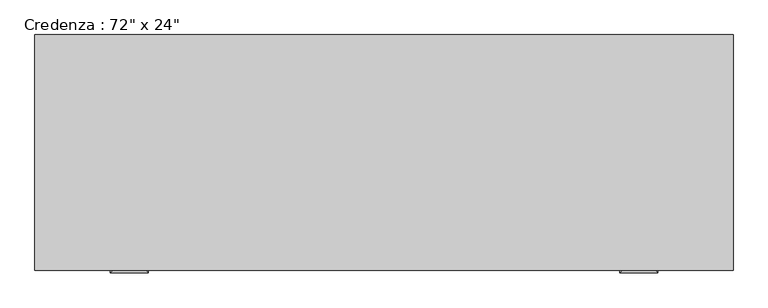
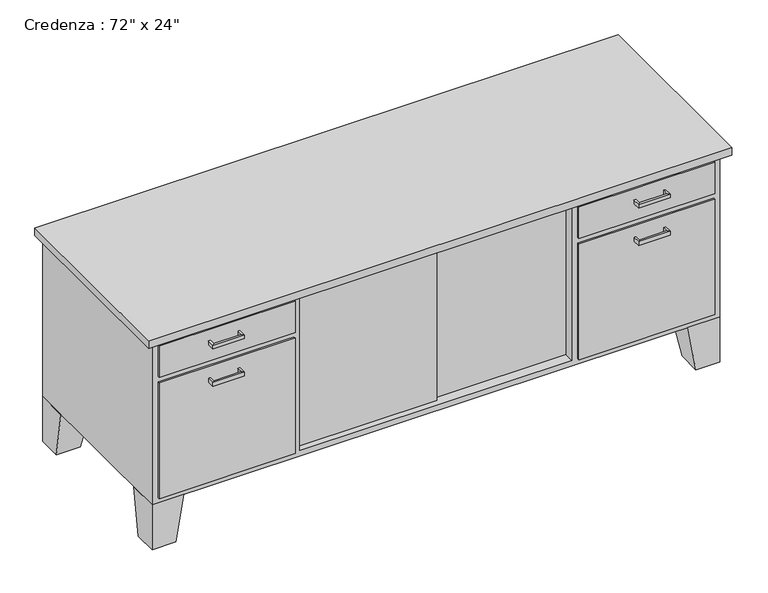
"""IFC4 building model written with IfcOpenShell, lengths in millimetres: furniture geometry."""

from ifc_helpers import new_model, si_unit, frame, origin, place, context, project, spatial, polyline, outline, extrude, faceted_brep, source, transform, mapped, element, save


def furniture_7b927048(model_context):
    return source(origin(), model_context, "Body", "SolidModel", [
        extrude(outline(polyline([(531.7023176, -267.2714583), (46.8442623, -267.2714583), (46.8442623, -254.5714583), (531.7023176, -254.5714583), (531.7023176, -267.2714583)])), frame((0.0, 0.0, 171.45), z_axis=(0.0, 0.0, 1.0), x_axis=(1.0, 0.0, 0.0)), (0.0, 0.0, 1.0), 520.7),
        extrude(outline(polyline([(73.6254475, -279.9714583), (-378.6057377, -279.9714583), (-378.6057377, -267.2714583), (73.6254475, -267.2714583), (73.6254475, -279.9714583)])), frame((0.0, 0.0, 171.45), z_axis=(0.0, 0.0, 1.0), x_axis=(1.0, 0.0, 0.0)), (0.0, 0.0, 1.0), 520.7),
        faceted_brep([(872.3442623, 309.3803279, 152.4), (872.3442623, 207.7803279, 152.4), (973.9442623, 207.7803279, 152.4), (973.9442623, 309.3803279, 152.4), (897.7442623, 309.3803279, 0.0), (973.9442623, 309.3803279, 0.0), (973.9442623, 233.1803279, 0.0), (897.7442623, 233.1803279, 0.0)], [[[0, 1, 2, 3]], [[4, 5, 6, 7]], [[4, 7, 1, 0]], [[7, 6, 2, 1]], [[6, 5, 3, 2]], [[5, 4, 0, 3]]]),
        extrude(outline(polyline([(954.8942623, -306.5696721), (516.7442623, -306.5696721), (516.7442623, -300.2196721), (954.8942623, -300.2196721), (954.8942623, -306.5696721)])), frame((0.0, 0.0, 584.2), z_axis=(0.0, 0.0, 1.0), x_axis=(1.0, 0.0, 0.0)), (0.0, 0.0, 1.0), 107.95),
        extrude(outline(polyline([(954.8942623, -306.5696721), (516.7442623, -306.5696721), (516.7442623, -300.2196721), (954.8942623, -300.2196721), (954.8942623, -306.5696721)])), frame((0.0, 0.0, 171.45), z_axis=(0.0, 0.0, 1.0), x_axis=(1.0, 0.0, 0.0)), (0.0, 0.0, 1.0), 393.7),
        extrude(outline(polyline([(-397.6557377, -306.5696721), (-835.8057377, -306.5696721), (-835.8057377, -300.2196721), (-397.6557377, -300.2196721), (-397.6557377, -306.5696721)])), frame((0.0, 0.0, 584.2), z_axis=(0.0, 0.0, 1.0), x_axis=(1.0, 0.0, 0.0)), (0.0, 0.0, 1.0), 107.95),
        extrude(outline(polyline([(-397.6557377, -306.5696721), (-835.8057377, -306.5696721), (-835.8057377, -300.2196721), (-397.6557377, -300.2196721), (-397.6557377, -306.5696721)])), frame((0.0, 0.0, 171.45), z_axis=(0.0, 0.0, 1.0), x_axis=(1.0, 0.0, 0.0)), (0.0, 0.0, 1.0), 393.7),
        faceted_brep([(-753.2557377, -300.2196721, 152.4), (-753.2557377, -198.6196721, 152.4), (-854.8557377, -198.6196721, 152.4), (-854.8557377, -300.2196721, 152.4), (-778.6557377, -300.2196721, 0.0), (-854.8557377, -300.2196721, 0.0), (-854.8557377, -224.0196721, 0.0), (-778.6557377, -224.0196721, 0.0)], [[[0, 1, 2, 3]], [[4, 5, 6, 7]], [[4, 7, 1, 0]], [[7, 6, 2, 1]], [[6, 5, 3, 2]], [[5, 4, 0, 3]]]),
        faceted_brep([(-753.2557377, 309.3803279, 152.4), (-854.8557377, 309.3803279, 152.4), (-854.8557377, 207.7803279, 152.4), (-753.2557377, 207.7803279, 152.4), (-778.6557377, 309.3803279, 0.0), (-778.6557377, 233.1803279, 0.0), (-854.8557377, 233.1803279, 0.0), (-854.8557377, 309.3803279, 0.0)], [[[0, 1, 2, 3]], [[4, 5, 6, 7]], [[4, 7, 1, 0]], [[7, 6, 2, 1]], [[6, 5, 3, 2]], [[5, 4, 0, 3]]]),
        faceted_brep([(872.3442623, -300.2196721, 152.4), (973.9442623, -300.2196721, 152.4), (973.9442623, -198.6196721, 152.4), (872.3442623, -198.6196721, 152.4), (897.7442623, -300.2196721, 0.0), (897.7442623, -224.0196721, 0.0), (973.9442623, -224.0196721, 0.0), (973.9442623, -300.2196721, 0.0)], [[[0, 1, 2, 3]], [[4, 5, 6, 7]], [[4, 7, 1, 0]], [[7, 6, 2, 1]], [[6, 5, 3, 2]], [[5, 4, 0, 3]]]),
        faceted_brep([(973.9442623, 309.3803279, 711.2), (-854.8557377, 309.3803279, 711.2), (-854.8557377, -300.2196721, 711.2), (973.9442623, -300.2196721, 711.2), (973.9442623, 309.3803279, 152.4), (973.9442623, -300.2196721, 152.4), (-854.8557377, -300.2196721, 152.4), (-854.8557377, 309.3803279, 152.4), (-378.6057377, -300.2196721, 692.15), (497.6942623, -300.2196721, 692.15), (497.6942623, -300.2196721, 171.45), (-378.6057377, -300.2196721, 171.45), (497.6942623, 290.3303279, 692.15), (-378.6057377, 290.3303279, 692.15), (-378.6057377, 290.3303279, 171.45), (497.6942623, 290.3303279, 171.45)], [[[0, 1, 2, 3]], [[4, 5, 6, 7]], [[1, 0, 4, 7]], [[2, 1, 7, 6]], [[3, 2, 6, 5], [8, 9, 10, 11]], [[0, 3, 5, 4]], [[12, 13, 14, 15]], [[13, 12, 9, 8]], [[14, 13, 8, 11]], [[15, 14, 11, 10]], [[12, 15, 10, 9]]]),
        extrude(outline(polyline([(999.3442623, 309.3803279), (999.3442623, -325.6196721), (-880.2557377, -325.6196721), (-880.2557377, 309.3803279), (999.3442623, 309.3803279)])), frame((0.0, 0.0, 711.2), z_axis=(0.0, 0.0, 1.0), x_axis=(1.0, 0.0, 0.0)), (0.0, 0.0, 1.0), 25.4),
        faceted_brep([(-670.7057377, -306.5696721, 527.05), (-670.7057377, -306.5696721, 514.35), (-677.0557377, -306.5696721, 514.35), (-677.0557377, -306.5696721, 527.05), (-670.7057377, -325.6196721, 527.05), (-670.7057377, -325.6196721, 514.35), (-677.0557377, -331.9696721, 514.35), (-677.0557377, -331.9696721, 527.05), (-581.8057377, -325.6196721, 527.05), (-581.8057377, -325.6196721, 514.35), (-575.4557377, -331.9696721, 514.35), (-575.4557377, -331.9696721, 527.05), (-581.8057377, -306.5696721, 527.05), (-575.4557377, -306.5696721, 527.05), (-575.4557377, -306.5696721, 514.35), (-581.8057377, -306.5696721, 514.35)], [[[0, 1, 2, 3]], [[1, 0, 4, 5]], [[2, 1, 5, 6]], [[3, 2, 6, 7]], [[0, 3, 7, 4]], [[5, 4, 8, 9]], [[6, 5, 9, 10]], [[7, 6, 10, 11]], [[4, 7, 11, 8]], [[12, 13, 14, 15]], [[9, 8, 12, 15]], [[10, 9, 15, 14]], [[11, 10, 14, 13]], [[8, 11, 13, 12]]]),
        faceted_brep([(-670.7057377, -306.5696721, 654.05), (-670.7057377, -306.5696721, 641.35), (-677.0557377, -306.5696721, 641.35), (-677.0557377, -306.5696721, 654.05), (-670.7057377, -325.6196721, 654.05), (-670.7057377, -325.6196721, 641.35), (-677.0557377, -331.9696721, 641.35), (-677.0557377, -331.9696721, 654.05), (-581.8057377, -325.6196721, 654.05), (-581.8057377, -325.6196721, 641.35), (-575.4557377, -331.9696721, 641.35), (-575.4557377, -331.9696721, 654.05), (-581.8057377, -306.5696721, 654.05), (-575.4557377, -306.5696721, 654.05), (-575.4557377, -306.5696721, 641.35), (-581.8057377, -306.5696721, 641.35)], [[[0, 1, 2, 3]], [[1, 0, 4, 5]], [[2, 1, 5, 6]], [[3, 2, 6, 7]], [[0, 3, 7, 4]], [[5, 4, 8, 9]], [[6, 5, 9, 10]], [[7, 6, 10, 11]], [[4, 7, 11, 8]], [[12, 13, 14, 15]], [[9, 8, 12, 15]], [[10, 9, 15, 14]], [[11, 10, 14, 13]], [[8, 11, 13, 12]]]),
        faceted_brep([(700.8942623, -306.5696721, 654.1373112), (700.8942623, -306.5696721, 641.4373112), (694.5442623, -306.5696721, 641.4373112), (694.5442623, -306.5696721, 654.1373112), (700.8942623, -325.6196721, 654.1373112), (700.8942623, -325.6196721, 641.4373112), (694.5442623, -331.9696721, 641.4373112), (694.5442623, -331.9696721, 654.1373112), (789.7942623, -325.6196721, 654.1373112), (789.7942623, -325.6196721, 641.4373112), (796.1442623, -331.9696721, 641.4373112), (796.1442623, -331.9696721, 654.1373112), (789.7942623, -306.5696721, 654.1373112), (796.1442623, -306.5696721, 654.1373112), (796.1442623, -306.5696721, 641.4373112), (789.7942623, -306.5696721, 641.4373112)], [[[0, 1, 2, 3]], [[1, 0, 4, 5]], [[2, 1, 5, 6]], [[3, 2, 6, 7]], [[0, 3, 7, 4]], [[5, 4, 8, 9]], [[6, 5, 9, 10]], [[7, 6, 10, 11]], [[4, 7, 11, 8]], [[12, 13, 14, 15]], [[9, 8, 12, 15]], [[10, 9, 15, 14]], [[11, 10, 14, 13]], [[8, 11, 13, 12]]]),
        faceted_brep([(700.8942623, -306.5696721, 527.05), (700.8942623, -306.5696721, 514.35), (694.5442623, -306.5696721, 514.35), (694.5442623, -306.5696721, 527.05), (700.8942623, -325.6196721, 527.05), (700.8942623, -325.6196721, 514.35), (694.5442623, -331.9696721, 514.35), (694.5442623, -331.9696721, 527.05), (789.7942623, -325.6196721, 527.05), (789.7942623, -325.6196721, 514.35), (796.1442623, -331.9696721, 514.35), (796.1442623, -331.9696721, 527.05), (789.7942623, -306.5696721, 527.05), (796.1442623, -306.5696721, 527.05), (796.1442623, -306.5696721, 514.35), (789.7942623, -306.5696721, 514.35)], [[[0, 1, 2, 3]], [[1, 0, 4, 5]], [[2, 1, 5, 6]], [[3, 2, 6, 7]], [[0, 3, 7, 4]], [[5, 4, 8, 9]], [[6, 5, 9, 10]], [[7, 6, 10, 11]], [[4, 7, 11, 8]], [[12, 13, 14, 15]], [[9, 8, 12, 15]], [[10, 9, 15, 14]], [[11, 10, 14, 13]], [[8, 11, 13, 12]]]),
    ])


if __name__ == "__main__":
    model = new_model("IFC4")
    model_context = context("Model", 3, world=origin())
    ifc_project = project(units=[si_unit("LENGTHUNIT", "METRE", prefix="MILLI")], contexts=[model_context])
    site = spatial("IfcSite", under=ifc_project)
    building = spatial("IfcBuilding", under=site)
    placement = place(None, origin())
    furniture_shape = furniture_7b927048(model_context)
    element("IfcFurniture", 1, ObjectType="Credenza : 72\" x 24\"", at=placement, inside=building, context=model_context, shape_type="MappedRepresentation", body=[
        mapped(furniture_shape, transform((0.0, 0.0, 0.0), x_axis=(1.0, 0.0, 0.0), y_axis=(0.0, 1.0, 0.0), z_axis=(0.0, 0.0, 1.0))),
    ])
    save(model, "model.ifc")

# Revit data of these elements
# Type "Credenza : 72\" x 24\""
#   Assembly Code = "E2020200"
#   Depth = 2' - 0"
#   Height = 2' - 5"
#   Width = 6' - 0"
#   Body Material = Laminate, Ivory, Matte
#   Handles/Legs Material = Steel, Chrome Plated
#   Top Material = Cherry
#   Default Elevation = 0
# Element 1 (IfcFurniture, "Credenza : 72\" x 24\"")
#   Materials on its faces: "Steel, Chrome Plated", "Laminate, Ivory, Matte", "Cherry"
# Materials
#   "Laminate, Ivory, Matte": class "Plastic", colour RGB 247 247 239, transparency 0, Description = "Plastic Laminate - Ivory, Matte", Cost = 0
#   "Steel, Chrome Plated": class "Metal", colour RGB 17 17 17, transparency 0, Description = "Chromiuim plated steel", Cost = 0
#   "Cherry": class "Wood", colour RGB 226 177 128, transparency 0, Description = "Prunus Serotina", Cost = 0
